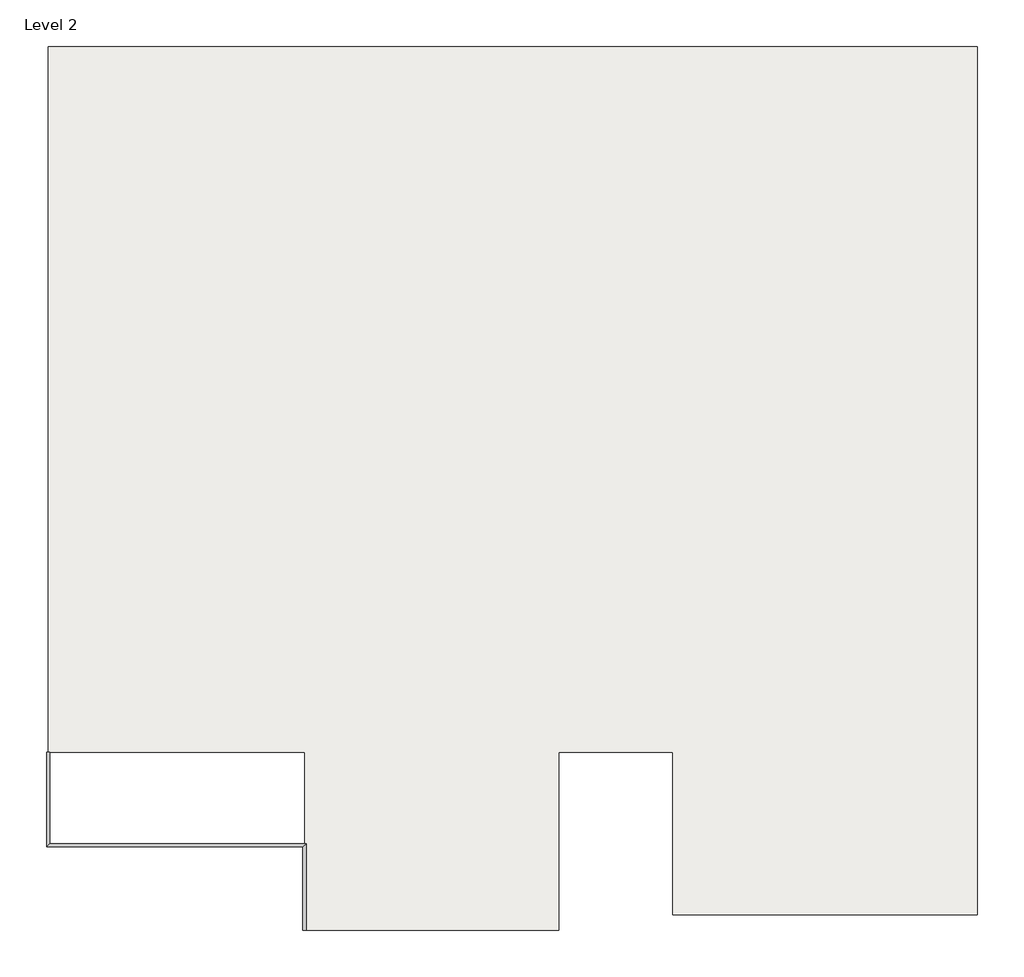
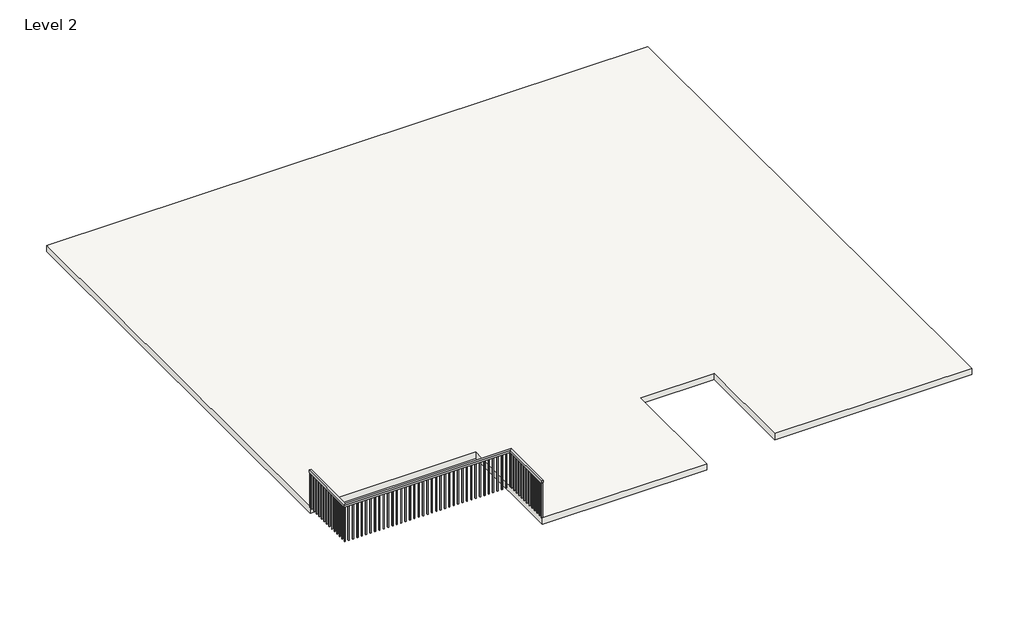
# One storey: 1 railing, 1 slab.
"""IFC4 building model written with IfcOpenShell, lengths in millimetres."""

from ifc_helpers import new_model, si_unit, frame, origin, place, context, project, spatial, polyline, outline, extrude, faceted_brep, element, save

model = new_model("IFC4")

# Units and contexts
model_context = context("Model", 3, world=origin())
ifc_project = project(units=[si_unit("LENGTHUNIT", "METRE", prefix="MILLI")], contexts=[model_context])

# Site, building, storey
site = spatial("IfcSite", under=ifc_project)
building = spatial("IfcBuilding", under=site)
storey = spatial("IfcBuildingStorey", under=building, Name="Level 2", Elevation=3657.6)

# Railing
placement = place(None, origin())
element("IfcRailing", 1, ObjectType="Handrail - Rectangular", at=placement, inside=storey, context=model_context, shape_type="SolidModel", body=[
    faceted_brep([(-2564.2864268, -714.3469744, 4673.6), (-2564.2864268, -714.3469744, 4724.4), (-6412.3864268, -714.3469744, 4724.4), (-6412.3864268, -714.3469744, 4673.6), (-2513.4864268, -663.5469744, 4673.6), (-6361.5864268, -663.5469744, 4673.6), (-2513.4864268, -663.5469744, 4724.4), (-6361.5864268, -663.5469744, 4724.4), (-6412.3864268, 705.2765264, 4724.4), (-6361.5864268, 705.2765264, 4724.4), (-6361.5864268, 705.2765264, 4673.6), (-6412.3864268, 705.2765264, 4673.6), (-2564.2864268, -1961.7234736, 4724.4), (-2564.2864268, -1961.7234736, 4673.6), (-2513.4864268, -1961.7234736, 4673.6), (-2513.4864268, -1961.7234736, 4724.4)], [[[0, 1, 2, 3]], [[4, 0, 3, 5]], [[6, 4, 5, 7]], [[1, 6, 7, 2]], [[8, 9, 10, 11]], [[3, 2, 8, 11]], [[5, 3, 11, 10]], [[7, 5, 10, 9]], [[2, 7, 9, 8]], [[12, 13, 14, 15]], [[13, 12, 1, 0]], [[14, 13, 0, 4]], [[15, 14, 4, 6]], [[12, 15, 6, 1]]]),
    extrude(outline(polyline([(-6377.4614268, 622.3280256), (-6396.5114268, 622.3280256), (-6396.5114268, 641.3780256), (-6377.4614268, 641.3780256), (-6377.4614268, 622.3280256)])), frame((0.0, 0.0, 3810.0), z_axis=(0.0, 0.0, 1.0), x_axis=(1.0, 0.0, 0.0)), (0.0, 0.0, 1.0), 863.6),
    extrude(outline(polyline([(-6377.4614268, 520.7280256), (-6396.5114268, 520.7280256), (-6396.5114268, 539.7780256), (-6377.4614268, 539.7780256), (-6377.4614268, 520.7280256)])), frame((0.0, 0.0, 3810.0), z_axis=(0.0, 0.0, 1.0), x_axis=(1.0, 0.0, 0.0)), (0.0, 0.0, 1.0), 863.6),
    extrude(outline(polyline([(-6377.4614268, 419.1280256), (-6396.5114268, 419.1280256), (-6396.5114268, 438.1780256), (-6377.4614268, 438.1780256), (-6377.4614268, 419.1280256)])), frame((0.0, 0.0, 3810.0), z_axis=(0.0, 0.0, 1.0), x_axis=(1.0, 0.0, 0.0)), (0.0, 0.0, 1.0), 863.6),
    extrude(outline(polyline([(-6377.4614268, 317.5280256), (-6396.5114268, 317.5280256), (-6396.5114268, 336.5780256), (-6377.4614268, 336.5780256), (-6377.4614268, 317.5280256)])), frame((0.0, 0.0, 3810.0), z_axis=(0.0, 0.0, 1.0), x_axis=(1.0, 0.0, 0.0)), (0.0, 0.0, 1.0), 863.6),
    extrude(outline(polyline([(-6377.4614268, 215.9280256), (-6396.5114268, 215.9280256), (-6396.5114268, 234.9780256), (-6377.4614268, 234.9780256), (-6377.4614268, 215.9280256)])), frame((0.0, 0.0, 3810.0), z_axis=(0.0, 0.0, 1.0), x_axis=(1.0, 0.0, 0.0)), (0.0, 0.0, 1.0), 863.6),
    extrude(outline(polyline([(-6377.4614268, 114.3280256), (-6396.5114268, 114.3280256), (-6396.5114268, 133.3780256), (-6377.4614268, 133.3780256), (-6377.4614268, 114.3280256)])), frame((0.0, 0.0, 3810.0), z_axis=(0.0, 0.0, 1.0), x_axis=(1.0, 0.0, 0.0)), (0.0, 0.0, 1.0), 863.6),
    extrude(outline(polyline([(-6377.4614268, 12.7280256), (-6396.5114268, 12.7280256), (-6396.5114268, 31.7780256), (-6377.4614268, 31.7780256), (-6377.4614268, 12.7280256)])), frame((0.0, 0.0, 3810.0), z_axis=(0.0, 0.0, 1.0), x_axis=(1.0, 0.0, 0.0)), (0.0, 0.0, 1.0), 863.6),
    extrude(outline(polyline([(-6377.4614268, -88.8719744), (-6396.5114268, -88.8719744), (-6396.5114268, -69.8219744), (-6377.4614268, -69.8219744), (-6377.4614268, -88.8719744)])), frame((0.0, 0.0, 3810.0), z_axis=(0.0, 0.0, 1.0), x_axis=(1.0, 0.0, 0.0)), (0.0, 0.0, 1.0), 863.6),
    extrude(outline(polyline([(-6377.4614268, -190.4719744), (-6396.5114268, -190.4719744), (-6396.5114268, -171.4219744), (-6377.4614268, -171.4219744), (-6377.4614268, -190.4719744)])), frame((0.0, 0.0, 3810.0), z_axis=(0.0, 0.0, 1.0), x_axis=(1.0, 0.0, 0.0)), (0.0, 0.0, 1.0), 863.6),
    extrude(outline(polyline([(-6377.4614268, -292.0719744), (-6396.5114268, -292.0719744), (-6396.5114268, -273.0219744), (-6377.4614268, -273.0219744), (-6377.4614268, -292.0719744)])), frame((0.0, 0.0, 3810.0), z_axis=(0.0, 0.0, 1.0), x_axis=(1.0, 0.0, 0.0)), (0.0, 0.0, 1.0), 863.6),
    extrude(outline(polyline([(-6377.4614268, -393.6719744), (-6396.5114268, -393.6719744), (-6396.5114268, -374.6219744), (-6377.4614268, -374.6219744), (-6377.4614268, -393.6719744)])), frame((0.0, 0.0, 3810.0), z_axis=(0.0, 0.0, 1.0), x_axis=(1.0, 0.0, 0.0)), (0.0, 0.0, 1.0), 863.6),
    extrude(outline(polyline([(-6377.4614268, -495.2719744), (-6396.5114268, -495.2719744), (-6396.5114268, -476.2219744), (-6377.4614268, -476.2219744), (-6377.4614268, -495.2719744)])), frame((0.0, 0.0, 3810.0), z_axis=(0.0, 0.0, 1.0), x_axis=(1.0, 0.0, 0.0)), (0.0, 0.0, 1.0), 863.6),
    extrude(outline(polyline([(-6377.4614268, -596.8719744), (-6396.5114268, -596.8719744), (-6396.5114268, -577.8219744), (-6377.4614268, -577.8219744), (-6377.4614268, -596.8719744)])), frame((0.0, 0.0, 3810.0), z_axis=(0.0, 0.0, 1.0), x_axis=(1.0, 0.0, 0.0)), (0.0, 0.0, 1.0), 863.6),
    extrude(outline(polyline([(-6288.5614268, -679.4219744), (-6288.5614268, -698.4719744), (-6307.6114268, -698.4719744), (-6307.6114268, -679.4219744), (-6288.5614268, -679.4219744)])), frame((0.0, 0.0, 3810.0), z_axis=(0.0, 0.0, 1.0), x_axis=(1.0, 0.0, 0.0)), (0.0, 0.0, 1.0), 863.6),
    extrude(outline(polyline([(-6186.9614268, -679.4219744), (-6186.9614268, -698.4719744), (-6206.0114268, -698.4719744), (-6206.0114268, -679.4219744), (-6186.9614268, -679.4219744)])), frame((0.0, 0.0, 3810.0), z_axis=(0.0, 0.0, 1.0), x_axis=(1.0, 0.0, 0.0)), (0.0, 0.0, 1.0), 863.6),
    extrude(outline(polyline([(-6085.3614268, -679.4219744), (-6085.3614268, -698.4719744), (-6104.4114268, -698.4719744), (-6104.4114268, -679.4219744), (-6085.3614268, -679.4219744)])), frame((0.0, 0.0, 3810.0), z_axis=(0.0, 0.0, 1.0), x_axis=(1.0, 0.0, 0.0)), (0.0, 0.0, 1.0), 863.6),
    extrude(outline(polyline([(-5983.7614268, -679.4219744), (-5983.7614268, -698.4719744), (-6002.8114268, -698.4719744), (-6002.8114268, -679.4219744), (-5983.7614268, -679.4219744)])), frame((0.0, 0.0, 3810.0), z_axis=(0.0, 0.0, 1.0), x_axis=(1.0, 0.0, 0.0)), (0.0, 0.0, 1.0), 863.6),
    extrude(outline(polyline([(-5882.1614268, -679.4219744), (-5882.1614268, -698.4719744), (-5901.2114268, -698.4719744), (-5901.2114268, -679.4219744), (-5882.1614268, -679.4219744)])), frame((0.0, 0.0, 3810.0), z_axis=(0.0, 0.0, 1.0), x_axis=(1.0, 0.0, 0.0)), (0.0, 0.0, 1.0), 863.6),
    extrude(outline(polyline([(-5780.5614268, -679.4219744), (-5780.5614268, -698.4719744), (-5799.6114268, -698.4719744), (-5799.6114268, -679.4219744), (-5780.5614268, -679.4219744)])), frame((0.0, 0.0, 3810.0), z_axis=(0.0, 0.0, 1.0), x_axis=(1.0, 0.0, 0.0)), (0.0, 0.0, 1.0), 863.6),
    extrude(outline(polyline([(-5678.9614268, -679.4219744), (-5678.9614268, -698.4719744), (-5698.0114268, -698.4719744), (-5698.0114268, -679.4219744), (-5678.9614268, -679.4219744)])), frame((0.0, 0.0, 3810.0), z_axis=(0.0, 0.0, 1.0), x_axis=(1.0, 0.0, 0.0)), (0.0, 0.0, 1.0), 863.6),
    extrude(outline(polyline([(-5577.3614268, -679.4219744), (-5577.3614268, -698.4719744), (-5596.4114268, -698.4719744), (-5596.4114268, -679.4219744), (-5577.3614268, -679.4219744)])), frame((0.0, 0.0, 3810.0), z_axis=(0.0, 0.0, 1.0), x_axis=(1.0, 0.0, 0.0)), (0.0, 0.0, 1.0), 863.6),
    extrude(outline(polyline([(-5475.7614268, -679.4219744), (-5475.7614268, -698.4719744), (-5494.8114268, -698.4719744), (-5494.8114268, -679.4219744), (-5475.7614268, -679.4219744)])), frame((0.0, 0.0, 3810.0), z_axis=(0.0, 0.0, 1.0), x_axis=(1.0, 0.0, 0.0)), (0.0, 0.0, 1.0), 863.6),
    extrude(outline(polyline([(-5374.1614268, -679.4219744), (-5374.1614268, -698.4719744), (-5393.2114268, -698.4719744), (-5393.2114268, -679.4219744), (-5374.1614268, -679.4219744)])), frame((0.0, 0.0, 3810.0), z_axis=(0.0, 0.0, 1.0), x_axis=(1.0, 0.0, 0.0)), (0.0, 0.0, 1.0), 863.6),
    extrude(outline(polyline([(-5272.5614268, -679.4219744), (-5272.5614268, -698.4719744), (-5291.6114268, -698.4719744), (-5291.6114268, -679.4219744), (-5272.5614268, -679.4219744)])), frame((0.0, 0.0, 3810.0), z_axis=(0.0, 0.0, 1.0), x_axis=(1.0, 0.0, 0.0)), (0.0, 0.0, 1.0), 863.6),
    extrude(outline(polyline([(-5170.9614268, -679.4219744), (-5170.9614268, -698.4719744), (-5190.0114268, -698.4719744), (-5190.0114268, -679.4219744), (-5170.9614268, -679.4219744)])), frame((0.0, 0.0, 3810.0), z_axis=(0.0, 0.0, 1.0), x_axis=(1.0, 0.0, 0.0)), (0.0, 0.0, 1.0), 863.6),
    extrude(outline(polyline([(-5069.3614268, -679.4219744), (-5069.3614268, -698.4719744), (-5088.4114268, -698.4719744), (-5088.4114268, -679.4219744), (-5069.3614268, -679.4219744)])), frame((0.0, 0.0, 3810.0), z_axis=(0.0, 0.0, 1.0), x_axis=(1.0, 0.0, 0.0)), (0.0, 0.0, 1.0), 863.6),
    extrude(outline(polyline([(-4967.7614268, -679.4219744), (-4967.7614268, -698.4719744), (-4986.8114268, -698.4719744), (-4986.8114268, -679.4219744), (-4967.7614268, -679.4219744)])), frame((0.0, 0.0, 3810.0), z_axis=(0.0, 0.0, 1.0), x_axis=(1.0, 0.0, 0.0)), (0.0, 0.0, 1.0), 863.6),
    extrude(outline(polyline([(-4866.1614268, -679.4219744), (-4866.1614268, -698.4719744), (-4885.2114268, -698.4719744), (-4885.2114268, -679.4219744), (-4866.1614268, -679.4219744)])), frame((0.0, 0.0, 3810.0), z_axis=(0.0, 0.0, 1.0), x_axis=(1.0, 0.0, 0.0)), (0.0, 0.0, 1.0), 863.6),
    extrude(outline(polyline([(-4764.5614268, -679.4219744), (-4764.5614268, -698.4719744), (-4783.6114268, -698.4719744), (-4783.6114268, -679.4219744), (-4764.5614268, -679.4219744)])), frame((0.0, 0.0, 3810.0), z_axis=(0.0, 0.0, 1.0), x_axis=(1.0, 0.0, 0.0)), (0.0, 0.0, 1.0), 863.6),
    extrude(outline(polyline([(-4662.9614268, -679.4219744), (-4662.9614268, -698.4719744), (-4682.0114268, -698.4719744), (-4682.0114268, -679.4219744), (-4662.9614268, -679.4219744)])), frame((0.0, 0.0, 3810.0), z_axis=(0.0, 0.0, 1.0), x_axis=(1.0, 0.0, 0.0)), (0.0, 0.0, 1.0), 863.6),
    extrude(outline(polyline([(-4561.3614268, -679.4219744), (-4561.3614268, -698.4719744), (-4580.4114268, -698.4719744), (-4580.4114268, -679.4219744), (-4561.3614268, -679.4219744)])), frame((0.0, 0.0, 3810.0), z_axis=(0.0, 0.0, 1.0), x_axis=(1.0, 0.0, 0.0)), (0.0, 0.0, 1.0), 863.6),
    extrude(outline(polyline([(-4459.7614268, -679.4219744), (-4459.7614268, -698.4719744), (-4478.8114268, -698.4719744), (-4478.8114268, -679.4219744), (-4459.7614268, -679.4219744)])), frame((0.0, 0.0, 3810.0), z_axis=(0.0, 0.0, 1.0), x_axis=(1.0, 0.0, 0.0)), (0.0, 0.0, 1.0), 863.6),
    extrude(outline(polyline([(-4358.1614268, -679.4219744), (-4358.1614268, -698.4719744), (-4377.2114268, -698.4719744), (-4377.2114268, -679.4219744), (-4358.1614268, -679.4219744)])), frame((0.0, 0.0, 3810.0), z_axis=(0.0, 0.0, 1.0), x_axis=(1.0, 0.0, 0.0)), (0.0, 0.0, 1.0), 863.6),
    extrude(outline(polyline([(-4256.5614268, -679.4219744), (-4256.5614268, -698.4719744), (-4275.6114268, -698.4719744), (-4275.6114268, -679.4219744), (-4256.5614268, -679.4219744)])), frame((0.0, 0.0, 3810.0), z_axis=(0.0, 0.0, 1.0), x_axis=(1.0, 0.0, 0.0)), (0.0, 0.0, 1.0), 863.6),
    extrude(outline(polyline([(-4154.9614268, -679.4219744), (-4154.9614268, -698.4719744), (-4174.0114268, -698.4719744), (-4174.0114268, -679.4219744), (-4154.9614268, -679.4219744)])), frame((0.0, 0.0, 3810.0), z_axis=(0.0, 0.0, 1.0), x_axis=(1.0, 0.0, 0.0)), (0.0, 0.0, 1.0), 863.6),
    extrude(outline(polyline([(-4053.3614268, -679.4219744), (-4053.3614268, -698.4719744), (-4072.4114268, -698.4719744), (-4072.4114268, -679.4219744), (-4053.3614268, -679.4219744)])), frame((0.0, 0.0, 3810.0), z_axis=(0.0, 0.0, 1.0), x_axis=(1.0, 0.0, 0.0)), (0.0, 0.0, 1.0), 863.6),
    extrude(outline(polyline([(-3951.7614268, -679.4219744), (-3951.7614268, -698.4719744), (-3970.8114268, -698.4719744), (-3970.8114268, -679.4219744), (-3951.7614268, -679.4219744)])), frame((0.0, 0.0, 3810.0), z_axis=(0.0, 0.0, 1.0), x_axis=(1.0, 0.0, 0.0)), (0.0, 0.0, 1.0), 863.6),
    extrude(outline(polyline([(-3850.1614268, -679.4219744), (-3850.1614268, -698.4719744), (-3869.2114268, -698.4719744), (-3869.2114268, -679.4219744), (-3850.1614268, -679.4219744)])), frame((0.0, 0.0, 3810.0), z_axis=(0.0, 0.0, 1.0), x_axis=(1.0, 0.0, 0.0)), (0.0, 0.0, 1.0), 863.6),
    extrude(outline(polyline([(-3748.5614268, -679.4219744), (-3748.5614268, -698.4719744), (-3767.6114268, -698.4719744), (-3767.6114268, -679.4219744), (-3748.5614268, -679.4219744)])), frame((0.0, 0.0, 3810.0), z_axis=(0.0, 0.0, 1.0), x_axis=(1.0, 0.0, 0.0)), (0.0, 0.0, 1.0), 863.6),
    extrude(outline(polyline([(-3646.9614268, -679.4219744), (-3646.9614268, -698.4719744), (-3666.0114268, -698.4719744), (-3666.0114268, -679.4219744), (-3646.9614268, -679.4219744)])), frame((0.0, 0.0, 3810.0), z_axis=(0.0, 0.0, 1.0), x_axis=(1.0, 0.0, 0.0)), (0.0, 0.0, 1.0), 863.6),
    extrude(outline(polyline([(-3545.3614268, -679.4219744), (-3545.3614268, -698.4719744), (-3564.4114268, -698.4719744), (-3564.4114268, -679.4219744), (-3545.3614268, -679.4219744)])), frame((0.0, 0.0, 3810.0), z_axis=(0.0, 0.0, 1.0), x_axis=(1.0, 0.0, 0.0)), (0.0, 0.0, 1.0), 863.6),
    extrude(outline(polyline([(-3443.7614268, -679.4219744), (-3443.7614268, -698.4719744), (-3462.8114268, -698.4719744), (-3462.8114268, -679.4219744), (-3443.7614268, -679.4219744)])), frame((0.0, 0.0, 3810.0), z_axis=(0.0, 0.0, 1.0), x_axis=(1.0, 0.0, 0.0)), (0.0, 0.0, 1.0), 863.6),
    extrude(outline(polyline([(-3342.1614268, -679.4219744), (-3342.1614268, -698.4719744), (-3361.2114268, -698.4719744), (-3361.2114268, -679.4219744), (-3342.1614268, -679.4219744)])), frame((0.0, 0.0, 3810.0), z_axis=(0.0, 0.0, 1.0), x_axis=(1.0, 0.0, 0.0)), (0.0, 0.0, 1.0), 863.6),
    extrude(outline(polyline([(-3240.5614268, -679.4219744), (-3240.5614268, -698.4719744), (-3259.6114268, -698.4719744), (-3259.6114268, -679.4219744), (-3240.5614268, -679.4219744)])), frame((0.0, 0.0, 3810.0), z_axis=(0.0, 0.0, 1.0), x_axis=(1.0, 0.0, 0.0)), (0.0, 0.0, 1.0), 863.6),
    extrude(outline(polyline([(-3138.9614268, -679.4219744), (-3138.9614268, -698.4719744), (-3158.0114268, -698.4719744), (-3158.0114268, -679.4219744), (-3138.9614268, -679.4219744)])), frame((0.0, 0.0, 3810.0), z_axis=(0.0, 0.0, 1.0), x_axis=(1.0, 0.0, 0.0)), (0.0, 0.0, 1.0), 863.6),
    extrude(outline(polyline([(-3037.3614268, -679.4219744), (-3037.3614268, -698.4719744), (-3056.4114268, -698.4719744), (-3056.4114268, -679.4219744), (-3037.3614268, -679.4219744)])), frame((0.0, 0.0, 3810.0), z_axis=(0.0, 0.0, 1.0), x_axis=(1.0, 0.0, 0.0)), (0.0, 0.0, 1.0), 863.6),
    extrude(outline(polyline([(-2935.7614268, -679.4219744), (-2935.7614268, -698.4719744), (-2954.8114268, -698.4719744), (-2954.8114268, -679.4219744), (-2935.7614268, -679.4219744)])), frame((0.0, 0.0, 3810.0), z_axis=(0.0, 0.0, 1.0), x_axis=(1.0, 0.0, 0.0)), (0.0, 0.0, 1.0), 863.6),
    extrude(outline(polyline([(-2834.1614268, -679.4219744), (-2834.1614268, -698.4719744), (-2853.2114268, -698.4719744), (-2853.2114268, -679.4219744), (-2834.1614268, -679.4219744)])), frame((0.0, 0.0, 3810.0), z_axis=(0.0, 0.0, 1.0), x_axis=(1.0, 0.0, 0.0)), (0.0, 0.0, 1.0), 863.6),
    extrude(outline(polyline([(-2732.5614268, -679.4219744), (-2732.5614268, -698.4719744), (-2751.6114268, -698.4719744), (-2751.6114268, -679.4219744), (-2732.5614268, -679.4219744)])), frame((0.0, 0.0, 3810.0), z_axis=(0.0, 0.0, 1.0), x_axis=(1.0, 0.0, 0.0)), (0.0, 0.0, 1.0), 863.6),
    extrude(outline(polyline([(-2630.9614268, -679.4219744), (-2630.9614268, -698.4719744), (-2650.0114268, -698.4719744), (-2650.0114268, -679.4219744), (-2630.9614268, -679.4219744)])), frame((0.0, 0.0, 3810.0), z_axis=(0.0, 0.0, 1.0), x_axis=(1.0, 0.0, 0.0)), (0.0, 0.0, 1.0), 863.6),
    extrude(outline(polyline([(-2529.3614268, -752.0484736), (-2548.4114268, -752.0484736), (-2548.4114268, -732.9984736), (-2529.3614268, -732.9984736), (-2529.3614268, -752.0484736)])), frame((0.0, 0.0, 3810.0), z_axis=(0.0, 0.0, 1.0), x_axis=(1.0, 0.0, 0.0)), (0.0, 0.0, 1.0), 863.6),
    extrude(outline(polyline([(-2529.3614268, -853.6484736), (-2548.4114268, -853.6484736), (-2548.4114268, -834.5984736), (-2529.3614268, -834.5984736), (-2529.3614268, -853.6484736)])), frame((0.0, 0.0, 3810.0), z_axis=(0.0, 0.0, 1.0), x_axis=(1.0, 0.0, 0.0)), (0.0, 0.0, 1.0), 863.6),
    extrude(outline(polyline([(-2529.3614268, -955.2484736), (-2548.4114268, -955.2484736), (-2548.4114268, -936.1984736), (-2529.3614268, -936.1984736), (-2529.3614268, -955.2484736)])), frame((0.0, 0.0, 3810.0), z_axis=(0.0, 0.0, 1.0), x_axis=(1.0, 0.0, 0.0)), (0.0, 0.0, 1.0), 863.6),
    extrude(outline(polyline([(-2529.3614268, -1056.8484736), (-2548.4114268, -1056.8484736), (-2548.4114268, -1037.7984736), (-2529.3614268, -1037.7984736), (-2529.3614268, -1056.8484736)])), frame((0.0, 0.0, 3810.0), z_axis=(0.0, 0.0, 1.0), x_axis=(1.0, 0.0, 0.0)), (0.0, 0.0, 1.0), 863.6),
    extrude(outline(polyline([(-2529.3614268, -1158.4484736), (-2548.4114268, -1158.4484736), (-2548.4114268, -1139.3984736), (-2529.3614268, -1139.3984736), (-2529.3614268, -1158.4484736)])), frame((0.0, 0.0, 3810.0), z_axis=(0.0, 0.0, 1.0), x_axis=(1.0, 0.0, 0.0)), (0.0, 0.0, 1.0), 863.6),
    extrude(outline(polyline([(-2529.3614268, -1260.0484736), (-2548.4114268, -1260.0484736), (-2548.4114268, -1240.9984736), (-2529.3614268, -1240.9984736), (-2529.3614268, -1260.0484736)])), frame((0.0, 0.0, 3810.0), z_axis=(0.0, 0.0, 1.0), x_axis=(1.0, 0.0, 0.0)), (0.0, 0.0, 1.0), 863.6),
    extrude(outline(polyline([(-2529.3614268, -1361.6484736), (-2548.4114268, -1361.6484736), (-2548.4114268, -1342.5984736), (-2529.3614268, -1342.5984736), (-2529.3614268, -1361.6484736)])), frame((0.0, 0.0, 3810.0), z_axis=(0.0, 0.0, 1.0), x_axis=(1.0, 0.0, 0.0)), (0.0, 0.0, 1.0), 863.6),
    extrude(outline(polyline([(-2529.3614268, -1463.2484736), (-2548.4114268, -1463.2484736), (-2548.4114268, -1444.1984736), (-2529.3614268, -1444.1984736), (-2529.3614268, -1463.2484736)])), frame((0.0, 0.0, 3810.0), z_axis=(0.0, 0.0, 1.0), x_axis=(1.0, 0.0, 0.0)), (0.0, 0.0, 1.0), 863.6),
    extrude(outline(polyline([(-2529.3614268, -1564.8484736), (-2548.4114268, -1564.8484736), (-2548.4114268, -1545.7984736), (-2529.3614268, -1545.7984736), (-2529.3614268, -1564.8484736)])), frame((0.0, 0.0, 3810.0), z_axis=(0.0, 0.0, 1.0), x_axis=(1.0, 0.0, 0.0)), (0.0, 0.0, 1.0), 863.6),
    extrude(outline(polyline([(-2529.3614268, -1666.4484736), (-2548.4114268, -1666.4484736), (-2548.4114268, -1647.3984736), (-2529.3614268, -1647.3984736), (-2529.3614268, -1666.4484736)])), frame((0.0, 0.0, 3810.0), z_axis=(0.0, 0.0, 1.0), x_axis=(1.0, 0.0, 0.0)), (0.0, 0.0, 1.0), 863.6),
    extrude(outline(polyline([(-2529.3614268, -1768.0484736), (-2548.4114268, -1768.0484736), (-2548.4114268, -1748.9984736), (-2529.3614268, -1748.9984736), (-2529.3614268, -1768.0484736)])), frame((0.0, 0.0, 3810.0), z_axis=(0.0, 0.0, 1.0), x_axis=(1.0, 0.0, 0.0)), (0.0, 0.0, 1.0), 863.6),
    extrude(outline(polyline([(-2529.3614268, -1869.6484736), (-2548.4114268, -1869.6484736), (-2548.4114268, -1850.5984736), (-2529.3614268, -1850.5984736), (-2529.3614268, -1869.6484736)])), frame((0.0, 0.0, 3810.0), z_axis=(0.0, 0.0, 1.0), x_axis=(1.0, 0.0, 0.0)), (0.0, 0.0, 1.0), 863.6),
    extrude(outline(polyline([(-6377.4614268, -679.4219744), (-6377.4614268, -698.4719744), (-6396.5114268, -698.4719744), (-6396.5114268, -679.4219744), (-6377.4614268, -679.4219744)])), frame((0.0, 0.0, 3810.0), z_axis=(0.0, 0.0, 1.0), x_axis=(1.0, 0.0, 0.0)), (0.0, 0.0, 1.0), 863.6),
    extrude(outline(polyline([(-2529.3614268, -698.4719744), (-2548.4114268, -698.4719744), (-2548.4114268, -679.4219744), (-2529.3614268, -679.4219744), (-2529.3614268, -698.4719744)])), frame((0.0, 0.0, 3810.0), z_axis=(0.0, 0.0, 1.0), x_axis=(1.0, 0.0, 0.0)), (0.0, 0.0, 1.0), 863.6),
    extrude(outline(polyline([(-6377.4614268, 686.2265264), (-6396.5114268, 686.2265264), (-6396.5114268, 705.2765264), (-6377.4614268, 705.2765264), (-6377.4614268, 686.2265264)])), frame((0.0, 0.0, 3810.0), z_axis=(0.0, 0.0, 1.0), x_axis=(1.0, 0.0, 0.0)), (0.0, 0.0, 1.0), 863.6),
    extrude(outline(polyline([(-2529.3614268, -1961.7234736), (-2548.4114268, -1961.7234736), (-2548.4114268, -1942.6734736), (-2529.3614268, -1942.6734736), (-2529.3614268, -1961.7234736)])), frame((0.0, 0.0, 3810.0), z_axis=(0.0, 0.0, 1.0), x_axis=(1.0, 0.0, 0.0)), (0.0, 0.0, 1.0), 863.6),
])

# Slab
element("IfcSlab", 2, ObjectType="6\" GF", at=placement, inside=storey, context=model_context, shape_type="SweptSolid", body=[
    extrude(outline(polyline([(-6386.9864268, 11297.0765264), (7557.6135732, 11297.0765264), (7557.6135732, -1733.1234736), (2985.6135732, -1733.1234736), (2985.6135732, 705.2765264), (1271.1135732, 705.2765264), (1271.1135732, -1961.7234736), (-2538.8864268, -1961.7234736), (-2538.8864268, 705.2765264), (-6386.9864268, 705.2765264), (-6386.9864268, 11297.0765264)])), frame((0.0, 0.0, 3657.6), z_axis=(0.0, 0.0, 1.0), x_axis=(1.0, 0.0, 0.0)), (0.0, 0.0, 1.0), 152.4),
])

save(model, "model.ifc")

# Revit data of these elements
# Type "Handrail - Rectangular"
#   Assembly Code = "C2010400"
#   built-in parameter 1008612 = 0.0416667 (stored number, unit not read)
#   built-in parameter 1008611 = 0.0416667 (stored number, unit not read)
#   built-in parameter 1008609 = 0.333333 (stored number, unit not read)
#   built-in parameter 1008604 = 0.166667 (stored number, unit not read)
#   built-in parameter 1008603 = 0.166667 (stored number, unit not read)
#   Railing Height = 3' - 0"
#   built-in parameter 1008630 = 2
#   built-in parameter 1008610 = 2
#   built-in parameter 1008618 = Baluster - Square : 3/4"
# Type "6\" GF"
#   Assembly Code = "B1010"
#   Function = 0
#   Layers, outside or top first: 0' - 6" "wall" (function 1)
# Element 1 (IfcRailing, "Handrail - Rectangular")
#   built-in parameter 1008621 = 0.5 (stored number, unit not read)
#   Phase Created = New Construction
# Element 2 (IfcSlab, "6\" GF")
#   built-in parameter 1001955 = 3.14159 (stored number, unit not read)
#   Height Offset From Level = 0' - 6"
#   Phase Created = New Construction
#   Materials on its faces: "wall"
# Materials
#   "wall": class "Generic", colour RGB 120 120 120, transparency 0, Cost = 0
